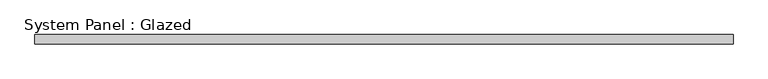
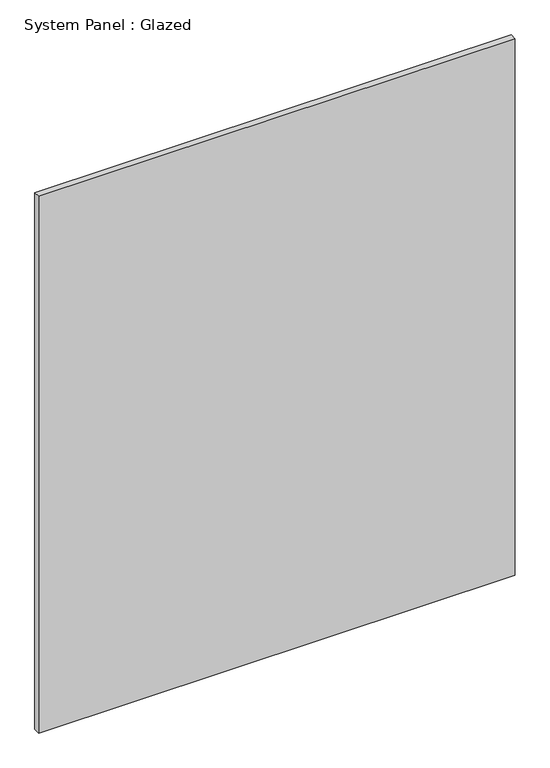
"""IFC4 building model written with IfcOpenShell, lengths in millimetres: plate geometry, System Panel : Glazed."""

from ifc_helpers import new_model, si_unit, origin, origin_with_axes, place, context, project, spatial, polyline, outline, extrude, source, transform, mapped, element, save


def system_panel_glazed_e26c2a08(model_context):
    return source(origin(), model_context, "Body", "SweptSolid", [
        extrude(outline(polyline([(945.4, 24.5), (-945.4, 24.5), (-945.4, 49.5), (945.4, 49.5), (945.4, 24.5)])), origin_with_axes(), (0.0, 0.0, 1.0), 2250.0),
    ])


if __name__ == "__main__":
    model = new_model("IFC4")
    model_context = context("Model", 3, world=origin())
    ifc_project = project(units=[si_unit("LENGTHUNIT", "METRE", prefix="MILLI")], contexts=[model_context])
    site = spatial("IfcSite", under=ifc_project)
    building = spatial("IfcBuilding", under=site)
    placement = place(None, origin())
    system_panel_glazed_shape = system_panel_glazed_e26c2a08(model_context)
    element("IfcPlate", 1, ObjectType="System Panel : Glazed", at=placement, inside=building, context=model_context, shape_type="MappedRepresentation", body=[
        mapped(system_panel_glazed_shape, transform((0.0, 0.0, 0.0), x_axis=(1.0, 0.0, 0.0), y_axis=(0.0, 1.0, 0.0), z_axis=(0.0, 0.0, 1.0))),
    ])
    save(model, "model.ifc")

# Revit data of these elements
# Type "System Panel : Glazed"
#   Keynote = "H11"
#   Construction Type Id = "GSP4R"
#   Analytic Construction = "1/8 in Pilkington single glazing"
#   Visual Light Transmittance = 0.9
#   Solar Heat Gain Coefficient = 0.86
#   Heat Transfer Coefficient (U) = 6.7069 W/(m²·K)
#   Define Thermal Properties by = 1
# Element 1 (IfcPlate, "System Panel : Glazed")
#   Materials on its faces: "Glass"
# Materials
#   "Glass": class "Glass", colour RGB 0 128 192, transparency 0.9, Description = "Soda Lime Glass", Cost = 0
